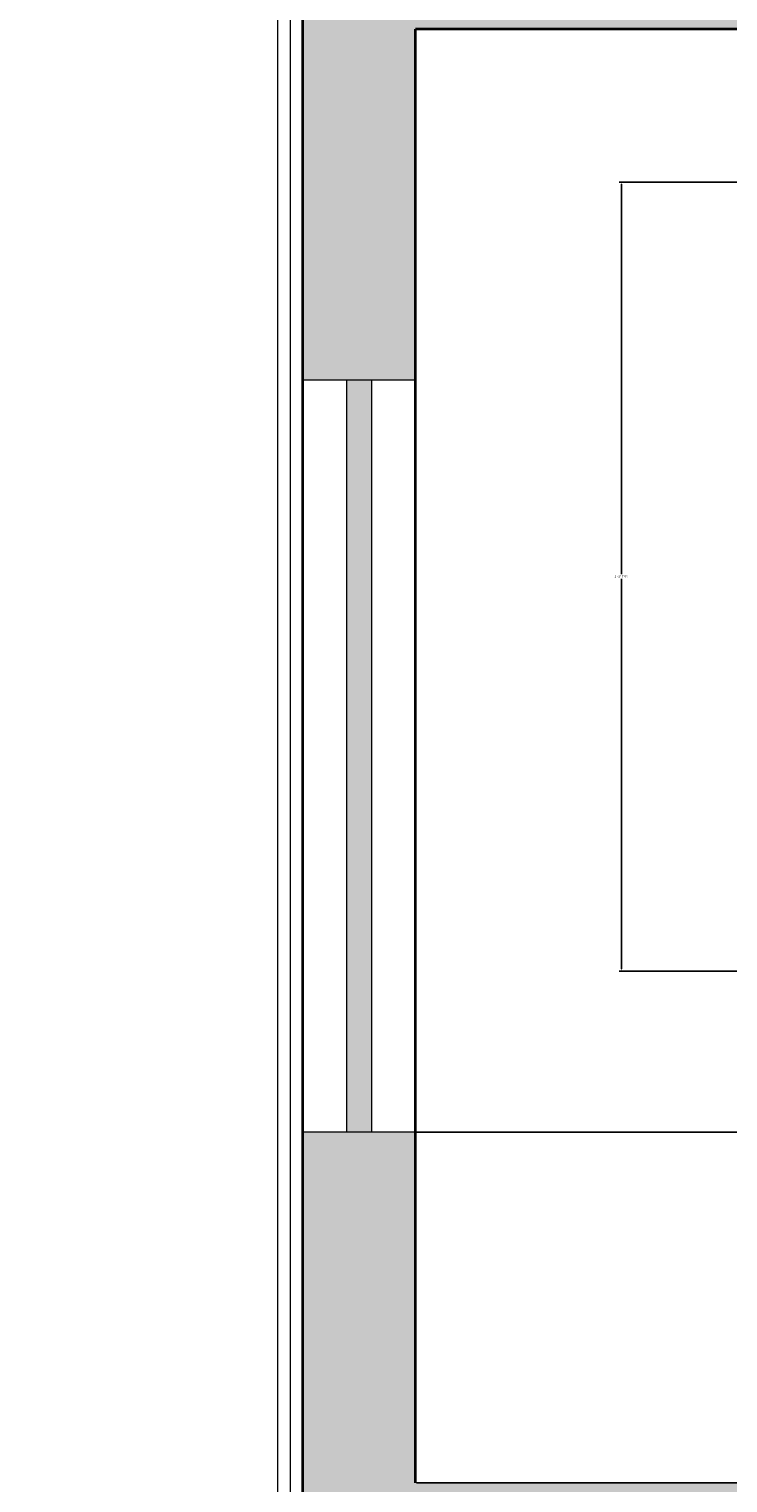
# Model space of a CAD drawing. Units: inches. Extents: x 311 to 815, y -527 to 136.
# Tile 17 of 21: x 388 to 444, y -103 to 13. Entities that reach past the tile are written whole.
import ezdxf

# ---------------------------------------------------------------- set-up
doc = ezdxf.new("R2010")
doc.units = ezdxf.units.IN
doc.header["$MEASUREMENT"] = 0
for name, color, linetype, lineweight in [('A-ANNO-DIMS', 1, 'Continuous', 18), ('A-FLOR-EDGE', 1, 'Continuous', 18), ('A-GLAZ-PATT', 5, 'Continuous', 13), ('A-WALL-PATT', 242, 'Continuous', 13), ('wall', 1, 'Continuous', 35), ('win', 5, 'Continuous', 18)]:
    doc.layers.add(name, color=color, linetype=linetype, lineweight=lineweight)
doc.styles.get("Standard").update_dxf_attribs({"font": 'arial.ttf'})
doc.dimstyles.get("Standard").update_dxf_attribs({"dimtxt": 0.18, "dimasz": 0.18, "dimexe": 0.18, "dimexo": 0.0625, "dimgap": 0.09, "dimtad": 0, "dimtih": 1, "dimtoh": 1, "dimdec": 1, "dimzin": 0, "dimdsep": 46, "dimlunit": 4, "dimtxsty": 'Standard', "dimcen": 0.09, "dimadec": 0, "dimazin": 0, "dimtfac": 1, "dimtdec": 1, "dimtofl": 0, "dimtmove": 0, "dimatfit": 3, "dimfxl": 1, "dimtolj": 1, "dimtzin": 0, "dimarcsym": 0})

# ---------------------------------------------------------------- blocks, each defined once
blk = doc.blocks.new('_ArchTick')
at = {"color": 0, "linetype": 'ByBlock', "const_width": 0.15}
blk.add_lwpolyline([(-0.5, -0.5), (0.5, 0.5)], dxfattribs=at)
blk = doc.blocks.new('_Oblique')
at = {"color": 0, "linetype": 'ByBlock', "lineweight": -2}
blk.add_line((-0.5, -0.5), (0.5, 0.5), dxfattribs=at)
blk = doc.blocks.new('*D3')
at = {"layer": 'A-ANNO-DIMS', "color": 0, "lineweight": -2, "transparency": 16777216}
for p, q in [((377.54, 21.87), (377.54, -221.61)), ((377.54, -482.13), (377.54, -238.65))]:
    blk.add_line(p, q, dxfattribs=at)
at = {"layer": 'Defpoints', "color": 0, "transparency": 16777216}
for p in [(410.32, 21.87), (377.54, -482.13), (410.32, -482.13)]:
    blk.add_point(p, dxfattribs=at)
at = {"layer": 'A-ANNO-DIMS', "color": 0, "lineweight": -2, "transparency": 16777216, "xscale": 9, "yscale": 9, "zscale": 9}
for name, p, rotation in [('_ArchTick', (377.54, 21.87), 90), ('_Oblique', (377.54, -482.13), 270)]:
    blk.add_blockref(name, p, dxfattribs=dict(at, rotation=rotation))
at = {"layer": 'A-ANNO-DIMS', "color": 0, "transparency": 16777216, "insert": (377.54, -230.13), "char_height": 9, "attachment_point": 5}
blk.add_mtext("\\A1;42'", dxfattribs=at)
blk = doc.blocks.new('WIN-60IN')
for p, q in [((9, 60), (0, 60)), ((3.5, 0), (3.5, 60)), ((5.5, 0), (5.5, 60)), ((9, 0), (0, 0))]:
    blk.add_line(p, q)
blk = doc.blocks.new('*D15')
at = {"layer": 'A-ANNO-DIMS', "color": 0, "lineweight": -2, "transparency": 16777216}
for p, q in [((445.75, 0.67), (435.57, 0.67)), ((435.75, 0.49), (435.75, -30.63)), ((435.75, -62.11), (435.75, -31)), ((445.75, -62.29), (435.57, -62.29))]:
    blk.add_line(p, q, dxfattribs=at)
at = {"layer": 'A-ANNO-DIMS', "color": 0, "transparency": 16777216}
for points in [[(435.72, 0.49), (435.78, 0.49), (435.75, 0.67)], [(435.72, -62.11), (435.78, -62.11), (435.75, -62.29)]]:
    blk.add_solid(points, dxfattribs=at)
at = {"layer": 'Defpoints', "color": 0, "transparency": 16777216}
for p in [(435.75, 0.67), (445.81, 0.67), (445.81, -62.29)]:
    blk.add_point(p, dxfattribs=at)
at = {"layer": 'A-ANNO-DIMS', "color": 0, "transparency": 16777216, "insert": (435.75, -30.81), "char_height": 0.18, "attachment_point": 5}
blk.add_mtext('\\A1;5\'-3" TYP.', dxfattribs=at)
blk = doc.blocks.new('*D40')
at = {"layer": 'A-ANNO-DIMS', "color": 0, "lineweight": -2, "transparency": 16777216}
for p, q in [((419.39, -75.13), (754.85, -75.13)), ((754.67, -75.31), (754.67, -88.95)), ((754.67, -102.95), (754.67, -89.31)), ((419.39, -103.13), (754.85, -103.13))]:
    blk.add_line(p, q, dxfattribs=at)
at = {"layer": 'A-ANNO-DIMS', "color": 0, "transparency": 16777216}
for points in [[(754.64, -75.31), (754.7, -75.31), (754.67, -75.13)], [(754.64, -102.95), (754.7, -102.95), (754.67, -103.13)]]:
    blk.add_solid(points, dxfattribs=at)
at = {"layer": 'Defpoints', "color": 0, "transparency": 16777216}
for p in [(419.32, -75.13), (419.32, -103.13), (754.67, -103.13)]:
    blk.add_point(p, dxfattribs=at)
at = {"layer": 'A-ANNO-DIMS', "color": 0, "transparency": 16777216, "insert": (754.67, -89.13), "char_height": 0.18, "attachment_point": 5}
blk.add_mtext('\\A1;2\'-4"', dxfattribs=at)

msp = doc.modelspace()

# ---------------------------------------------------------------- hatches: boundary and pattern name
at = {"layer": 'A-GLAZ-PATT'}
h = msp.add_hatch(color=256, dxfattribs=at)
h.dxf.hatch_style = 1
h.paths.add_polyline_path([(415.82, -15.13), (413.82, -15.13), (413.82, -75.13), (415.82, -75.13)])
h.paths.add_polyline_path([(415.82, -126.63), (413.82, -126.63), (413.82, -150.63), (415.82, -150.63)])
at = {"layer": 'A-WALL-PATT'}
h = msp.add_hatch(color=256, dxfattribs=at)
h.dxf.hatch_style = 1
h.paths.add_polyline_path([(557.82, 21.87), (509.32, 21.87), (509.32, 12.87), (539.32, 12.87), (539.32, -112.13), (548.32, -112.13), (548.32, -58.63), (557.82, -58.63), (557.82, -49.63), (548.32, -49.63), (548.32, 12.87), (557.82, 12.87)])
h.paths.add_polyline_path([(449.32, 21.87), (410.32, 21.87), (410.32, -15.13), (419.32, -15.13), (419.32, 12.87), (449.32, 12.87)])
h.paths.add_polyline_path([(626.82, 21.87), (581.82, 21.87), (581.82, 12.87), (591.32, 12.87), (591.32, -49.63), (581.82, -49.63), (581.82, -58.63), (591.32, -58.63), (591.32, -112.13), (600.32, -112.13), (600.32, 12.87), (626.82, 12.87)])
h.paths.add_polyline_path([(722.32, 21.87), (686.82, 21.87), (686.82, 12.87), (713.32, 12.87), (713.32, -18.13), (722.32, -18.13)])
h.paths.add_polyline_path([(722.32, -42.13), (713.32, -42.13), (713.32, -73.13), (722.32, -73.13)])
h.paths.add_polyline_path([(501.32, -103.13), (419.32, -103.13), (419.32, -75.13), (410.32, -75.13), (410.32, -126.63), (419.32, -126.63), (419.32, -112.13), (492.32, -112.13), (492.32, -143.13), (501.32, -143.13)])
h.paths.add_polyline_path([(548.32, -165.13), (419.32, -165.13), (419.32, -150.63), (410.32, -150.63), (410.32, -202.13), (419.32, -202.13), (419.32, -174.13), (548.32, -174.13)])
h.paths.add_polyline_path([(722.32, -103.13), (636.32, -103.13), (636.32, -112.13), (713.32, -112.13), (713.32, -140.13), (722.32, -140.13)])
h.paths.add_polyline_path([(548.32, -210.13), (539.32, -210.13), (539.32, -290.13), (419.32, -290.13), (419.32, -262.13), (410.32, -262.13), (410.32, -311.57), (419.32, -311.57), (419.32, -299.13), (469.32, -299.13), (469.32, -348.13), (443.32, -348.13), (443.32, -357.13), (478.32, -357.13), (478.32, -299.13), (548.32, -299.13)])
h.paths.add_polyline_path([(722.32, -200.13), (713.32, -200.13), (713.32, -228.13), (609.32, -228.13), (609.32, -237.13), (713.32, -237.13), (713.32, -262.63), (722.32, -262.63)])
h.paths.add_polyline_path([(722.32, -322.63), (713.32, -322.63), (713.32, -348.13), (633.32, -348.13), (633.32, -357.13), (713.32, -357.13), (713.32, -385.13), (722.32, -385.13)])
h.paths.add_polyline_path([(419.32, -335.57), (410.32, -335.57), (410.32, -390.84), (419.32, -390.84)])
h.paths.add_polyline_path([(419.32, -450.84), (410.32, -450.84), (410.32, -482.13), (449.32, -482.13), (449.32, -473.13), (419.32, -473.13)])
h.paths.add_polyline_path([(582.82, -473.13), (548.32, -473.13), (548.32, -348.13), (539.32, -348.13), (539.32, -473.13), (509.32, -473.13), (509.32, -482.13), (582.82, -482.13)])
h.paths.add_polyline_path([(722.32, -445.13), (713.32, -445.13), (713.32, -473.13), (678.82, -473.13), (678.82, -482.13), (722.32, -482.13)])

# ---------------------------------------------------------------- linework, layer by layer
at = {"layer": 'A-FLOR-EDGE'}
for p, q in [((408.32, -484.13), (408.32, 23.87)), ((409.32, -483.13), (409.32, 22.87))]:
    msp.add_line(p, q, dxfattribs=at)
at = {"layer": 'wall'}
for p, q in [((410.32, -482.13), (410.32, 21.87)), ((419.32, -103.13), (419.32, 12.87)), ((539.32, 12.87), (419.32, 12.87))]:
    msp.add_line(p, q, dxfattribs=at)

# ---------------------------------------------------------------- block references
at = {"layer": 'win'}
msp.add_blockref('WIN-60IN', (410.32, -75.13), dxfattribs=at)

# ---------------------------------------------------------------- dimensions: what is measured, and where the dimension line sits
at = {"layer": 'A-ANNO-DIMS'}
for base, p1, p2, override, picture, middle in [((377.54, -482.13), (410.32, 21.87), (410.32, -482.13), {"dimtxt": 9, "dimasz": 9, "dimgap": 4, "dimblk1": 'ArchTick', "dimblk2": 'Oblique', "dimsah": 1, "dimse1": 1, "dimse2": 1, "dimclrd": 0, "dimclre": 0, "dimclrt": 0}, '*D3', (377.54, -230.13)), ((754.67, -103.13), (419.32, -75.13), (419.32, -103.13), {"dimdec": 1, "dimlfac": 1, "dimrnd": 0, "dimzin": 1, "dimdsep": 46, "dimlunit": 4, "dimfrac": 2}, '*D40', (754.67, -89.13))]:
    dim = msp.add_linear_dim(base=base, p1=p1, p2=p2, angle=90, dimstyle='Standard', override=override, dxfattribs=at)
    dim.commit()
    dim.dimension.update_dxf_attribs({"geometry": picture, "text_midpoint": middle})
dim = msp.add_linear_dim(base=(435.75, 0.67), p1=(445.81, -62.29), p2=(445.81, 0.67), angle=90, text='<> TYP.', dimstyle='Standard', override={"dimdec": 1, "dimlfac": 1, "dimrnd": 0, "dimzin": 1, "dimdsep": 46, "dimlunit": 4, "dimfrac": 2}, dxfattribs=at)
dim.commit()
dim.dimension.update_dxf_attribs({"geometry": '*D15', "text_midpoint": (435.75, -30.81)})

doc.saveas('drawing.dxf')
